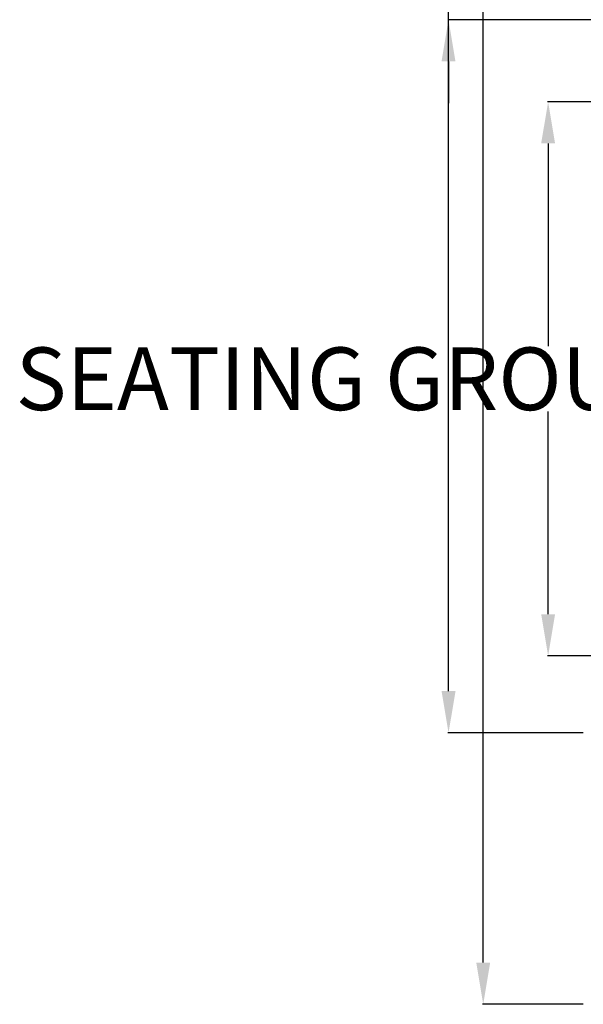
# Model space of a CAD drawing. Units: inches. Extents: x 2796 to 3603, y 978 to 1787.
# Tile 1 of 15: x 2908 to 3070, y 1029 to 1312. Entities that reach past the tile are written whole.
import ezdxf

# ---------------------------------------------------------------- set-up
doc = ezdxf.new("R2010")
doc.units = ezdxf.units.IN
doc.layers.add('A-ANNO-DIMS', color=7, linetype='Continuous', lineweight=18)
doc.styles.get("Standard").update_dxf_attribs({"font": 'arial.ttf'})
doc.dimstyles.get("Standard").update_dxf_attribs({"dimtxt": 18, "dimasz": 12, "dimexe": 0.18, "dimexo": 0.0625, "dimgap": 0.09, "dimtad": 0, "dimtih": 1, "dimtoh": 1, "dimdec": 0, "dimzin": 0, "dimdsep": 46, "dimlunit": 3, "dimtxsty": 'Standard', "dimcen": 0.09, "dimadec": 0, "dimazin": 0, "dimtfac": 1, "dimtdec": 0, "dimtofl": 0, "dimtmove": 0, "dimatfit": 3, "dimfxl": 1, "dimtolj": 1, "dimtzin": 0, "dimarcsym": 0})

# ---------------------------------------------------------------- blocks, each defined once
blk = doc.blocks.new('*D12')
at = {"layer": 'A-ANNO-DIMS', "color": 0, "lineweight": -2, "transparency": 16777216}
for p, q in [((3070.18, 1736.68), (3041.33, 1736.68)), ((3041.51, 1724.68), (3041.51, 1391.96)), ((3041.51, 1040.68), (3041.51, 1373.4)), ((3070.18, 1028.68), (3041.33, 1028.68))]:
    blk.add_line(p, q, dxfattribs=at)
at = {"layer": 'A-ANNO-DIMS', "color": 0, "transparency": 16777216}
for points in [[(3039.51, 1724.68), (3043.51, 1724.68), (3041.51, 1736.68)], [(3039.51, 1040.68), (3043.51, 1040.68), (3041.51, 1028.68)]]:
    blk.add_solid(points, dxfattribs=at)
at = {"layer": 'Defpoints', "color": 0, "transparency": 16777216}
for p in [(3041.51, 1736.68), (3070.25, 1736.68), (3070.25, 1028.68)]:
    blk.add_point(p, dxfattribs=at)
at = {"layer": 'A-ANNO-DIMS', "color": 0, "transparency": 16777216, "insert": (3041.51, 1382.68), "char_height": 18, "attachment_point": 5}
blk.add_mtext("\\A1;59'", dxfattribs=at)
blk = doc.blocks.new('*D30')
at = {"layer": 'A-ANNO-DIMS', "color": 0, "lineweight": -2, "transparency": 16777216}
for p, q in [((3083.98, 1288.1), (3059.97, 1288.1)), ((3060.15, 1276.1), (3060.15, 1217.86)), ((3060.15, 1140.81), (3060.15, 1199.05)), ((3083.98, 1128.81), (3059.97, 1128.81))]:
    blk.add_line(p, q, dxfattribs=at)
at = {"layer": 'A-ANNO-DIMS', "color": 0, "transparency": 16777216}
for points in [[(3058.15, 1276.1), (3062.15, 1276.1), (3060.15, 1288.1)], [(3058.15, 1140.81), (3062.15, 1140.81), (3060.15, 1128.81)]]:
    blk.add_solid(points, dxfattribs=at)
at = {"layer": 'Defpoints', "color": 0, "transparency": 16777216}
for p in [(3084.05, 1288.1), (3060.15, 1128.81), (3084.05, 1128.81)]:
    blk.add_point(p, dxfattribs=at)
at = {"layer": 'A-ANNO-DIMS', "color": 0, "transparency": 16777216, "insert": (3060.15, 1208.46), "char_height": 18, "attachment_point": 5}
blk.add_mtext('\\A1;SEATING GROUP 13\'-3 1/2"', dxfattribs=at)
blk = doc.blocks.new('*D45')
at = {"layer": 'A-ANNO-DIMS', "color": 0, "lineweight": -2, "transparency": 16777216}
for p, q in [((3070.18, 1736.68), (3031.37, 1736.68)), ((3031.55, 1724.68), (3031.55, 1430.96)), ((3031.55, 1118.68), (3031.55, 1412.4)), ((3070.18, 1106.68), (3031.37, 1106.68))]:
    blk.add_line(p, q, dxfattribs=at)
at = {"layer": 'A-ANNO-DIMS', "color": 0, "transparency": 16777216}
for points in [[(3029.55, 1724.68), (3033.55, 1724.68), (3031.55, 1736.68)], [(3029.55, 1118.68), (3033.55, 1118.68), (3031.55, 1106.68)]]:
    blk.add_solid(points, dxfattribs=at)
at = {"layer": 'Defpoints', "color": 0, "transparency": 16777216}
for p in [(3031.55, 1736.68), (3070.25, 1736.68), (3070.25, 1106.68)]:
    blk.add_point(p, dxfattribs=at)
at = {"layer": 'A-ANNO-DIMS', "color": 0, "transparency": 16777216, "insert": (3031.55, 1421.68), "char_height": 18, "attachment_point": 5}
blk.add_mtext('\\A1;52\'-6"', dxfattribs=at)
blk = doc.blocks.new('*D53')
at = {"layer": 'A-ANNO-DIMS', "color": 0, "lineweight": -2, "transparency": 16777216}
for p, q in [((3031.545499, 1347.67534), (3031.545499, 1359.67534)), ((3333.182999, 1335.67534), (3031.365499, 1335.67534)), ((3333.182999, 1311.67534), (3031.365499, 1311.67534)), ((3031.545499, 1299.67534), (3031.545499, 1287.67534))]:
    blk.add_line(p, q, dxfattribs=at)
at = {"layer": 'A-ANNO-DIMS', "color": 0, "transparency": 16777216}
for points in [[(3029.545499, 1347.67534), (3033.545499, 1347.67534), (3031.545499, 1335.67534)], [(3029.545499, 1299.67534), (3033.545499, 1299.67534), (3031.545499, 1311.67534)]]:
    blk.add_solid(points, dxfattribs=at)
at = {"layer": 'Defpoints', "color": 0, "transparency": 16777216}
for p in [(3031.545499, 1335.67534), (3333.245499, 1335.67534), (3333.245499, 1311.67534)]:
    blk.add_point(p, dxfattribs=at)
at = {"layer": 'A-ANNO-DIMS', "color": 0, "transparency": 16777216, "insert": (3031.545499, 1323.67534), "char_height": 18, "attachment_point": 5}
blk.add_mtext('\\A1;2\'-0"', dxfattribs=at)

msp = doc.modelspace()

# ---------------------------------------------------------------- dimensions: what is measured, and where the dimension line sits
at = {"layer": 'A-ANNO-DIMS'}
for base, p1, p2, override, picture, middle in [((3031.55, 1736.68), (3070.25, 1106.68), (3070.25, 1736.68), {"dimdec": 1, "dimlfac": 1, "dimrnd": 0, "dimzin": 1, "dimdsep": 46, "dimlunit": 4, "dimfrac": 2}, '*D45', (3031.55, 1421.68)), ((3041.51, 1736.68), (3070.25, 1028.68), (3070.25, 1736.68), {"dimclrd": 0, "dimclre": 0, "dimclrt": 0}, '*D12', (3041.51, 1382.68)), ((3031.55, 1335.68), (3333.25, 1311.68), (3333.25, 1335.68), {"dimdec": 1, "dimlfac": 1, "dimrnd": 0, "dimzin": 1, "dimdsep": 46, "dimlunit": 4, "dimfrac": 2}, '*D53', (3031.55, 1323.68))]:
    dim = msp.add_linear_dim(base=base, p1=p1, p2=p2, angle=90, dimstyle='Standard', override=override, dxfattribs=at)
    dim.commit()
    dim.dimension.update_dxf_attribs({"geometry": picture, "text_midpoint": middle})
dim = msp.add_linear_dim(base=(3060.15, 1128.81), p1=(3084.05, 1288.1), p2=(3084.05, 1128.81), angle=270, text='SEATING GROUP <>', dimstyle='Standard', override={"dimdec": 1, "dimlfac": 1, "dimrnd": 0, "dimzin": 1, "dimdsep": 46, "dimlunit": 4, "dimfrac": 2}, dxfattribs=at)
dim.commit()
dim.dimension.update_dxf_attribs({"geometry": '*D30', "text_midpoint": (3060.15, 1208.46)})

doc.saveas('drawing.dxf')
